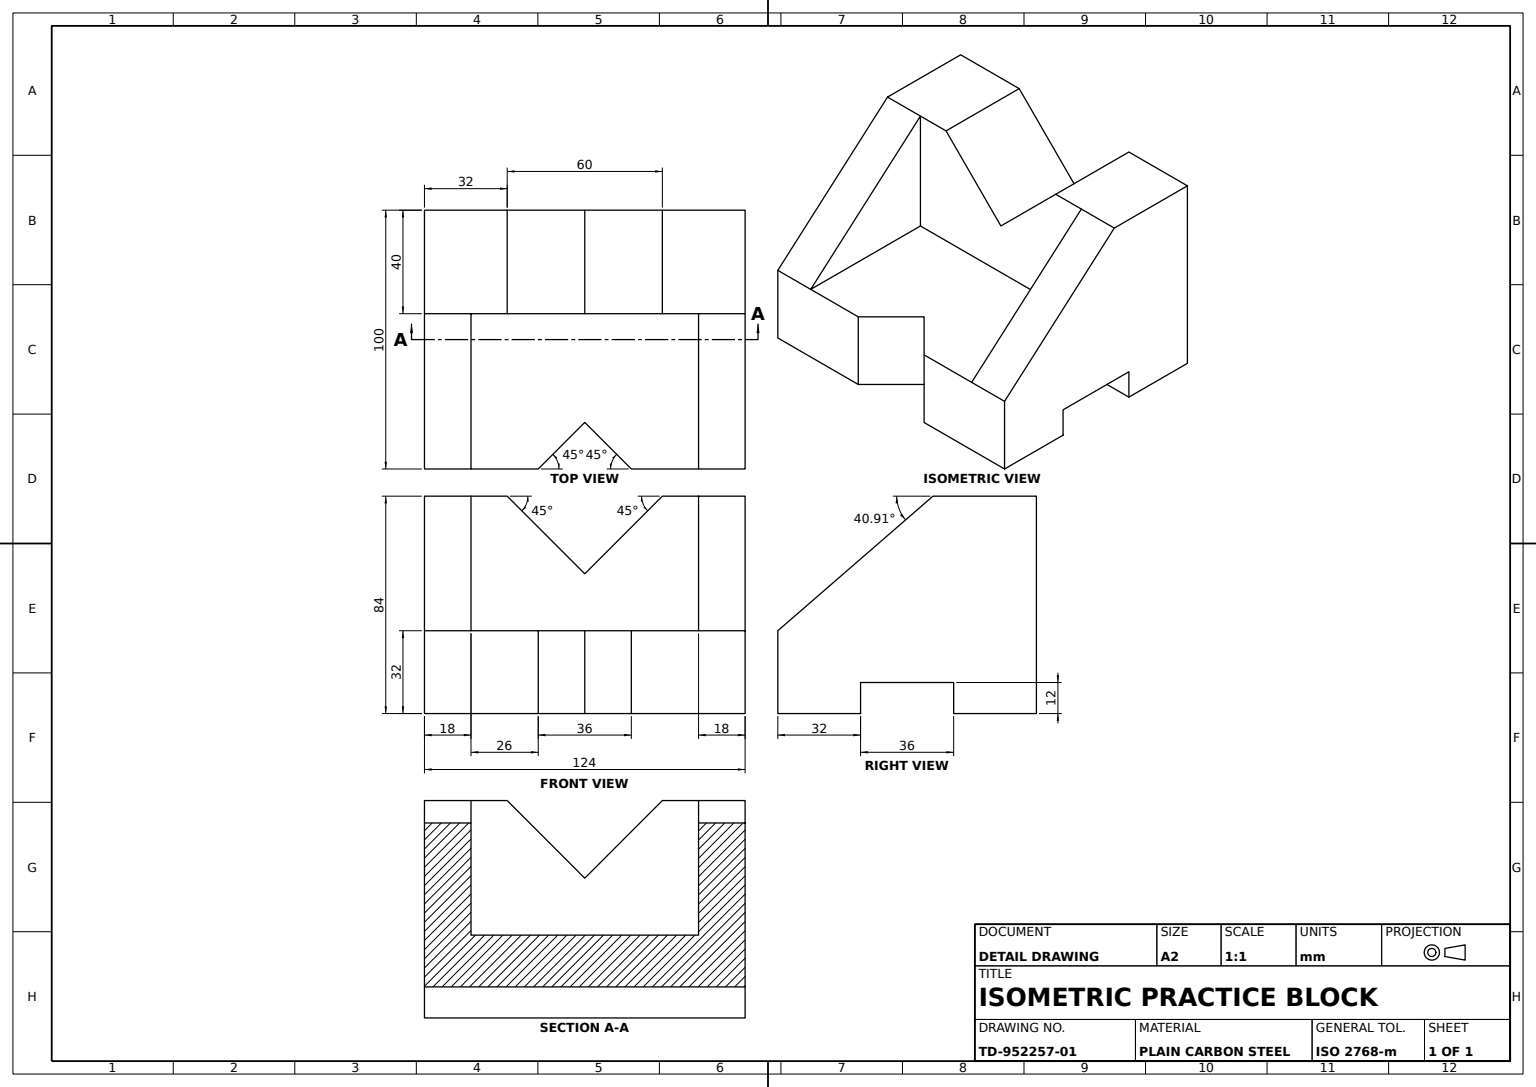
from build123d import *

# Parameters (mm, degrees)
SUPPORT_BLOCK_BODY_DEPTH    = 62
CENTRE_START                = 32
CENTRE_CHANNEL_SKETCH_W     = 60
CENTRE_CHANNEL_SKETCH_H     = 88
CENTRE_CHANNEL_CUT_DEPTH    = 124
V_NOTCH_CUT_DEPTH           = 124
BASE_GROOVE_CUT_18X36_REACH = 97.121
FRONT_NOTCH_CUT_REACH       = 159.899
FRONT_NOTCH_SKETCH_W        = 36
FRONT_NOTCH_SKETCH_H        = 12


with BuildPart() as part:
    # Block Profile Sketch → Support Block Body (new, symmetric)
    with BuildSketch(Plane.XY):
        Polygon((-50, 0), (50, 0), (50, 32), (-10, 84), (-50, 84), align=None)
    extrude(amount=SUPPORT_BLOCK_BODY_DEPTH, both=True)

    # Centre Channel Sketch → Centre Channel Cut (cut)
    with BuildSketch(Plane(origin=(0, 0, 0), x_dir=(1, 0, 0), z_dir=(0, 1, 0)).offset(CENTRE_START)):
        with Locations((20, 0)):
            Rectangle(CENTRE_CHANNEL_SKETCH_W, CENTRE_CHANNEL_SKETCH_H)
    extrude(amount=CENTRE_CHANNEL_CUT_DEPTH, mode=Mode.SUBTRACT)

    # V-Notch Sketch → V-Notch Cut (cut)
    with BuildSketch(Plane(origin=(-10, 0, 0), x_dir=(0, 0, -1), z_dir=(1, 0, 0))):
        Polygon((30, 84), (0, 54), (-30, 84), align=None)
    extrude(amount=-V_NOTCH_CUT_DEPTH, mode=Mode.SUBTRACT)

    # Base Groove Sketch → Base Groove Cut 18x36 (cut, up to next)
    with BuildSketch(Plane(origin=(0, 32, 0), x_dir=(1, 0, 0), z_dir=(0, 1, 0)), mode=Mode.PRIVATE) as base_groove_cut_18x36_sk1:
        Polygon((50, 18), (32, 0), (50, -18), align=None)
    base_groove_cut_18x36_tool1 = extrude(base_groove_cut_18x36_sk1.sketch, amount=-BASE_GROOVE_CUT_18X36_REACH, mode=Mode.PRIVATE) & part.part
    add(base_groove_cut_18x36_tool1.solids().sort_by_distance((44, 32, 0))[0], mode=Mode.SUBTRACT)

    # Front Notch Sketch → Front Notch Cut (cut, up to next)
    with BuildSketch(Plane.XY.offset(62), mode=Mode.PRIVATE) as front_notch_cut_sk1:
        with Locations((0, 6)):
            Rectangle(FRONT_NOTCH_SKETCH_W, FRONT_NOTCH_SKETCH_H)
    front_notch_cut_tool1 = extrude(front_notch_cut_sk1.sketch, amount=-FRONT_NOTCH_CUT_REACH, mode=Mode.PRIVATE) & part.part
    add(front_notch_cut_tool1.solids().sort_by_distance((0, 6, 62))[0], mode=Mode.SUBTRACT)


solid = part.part
